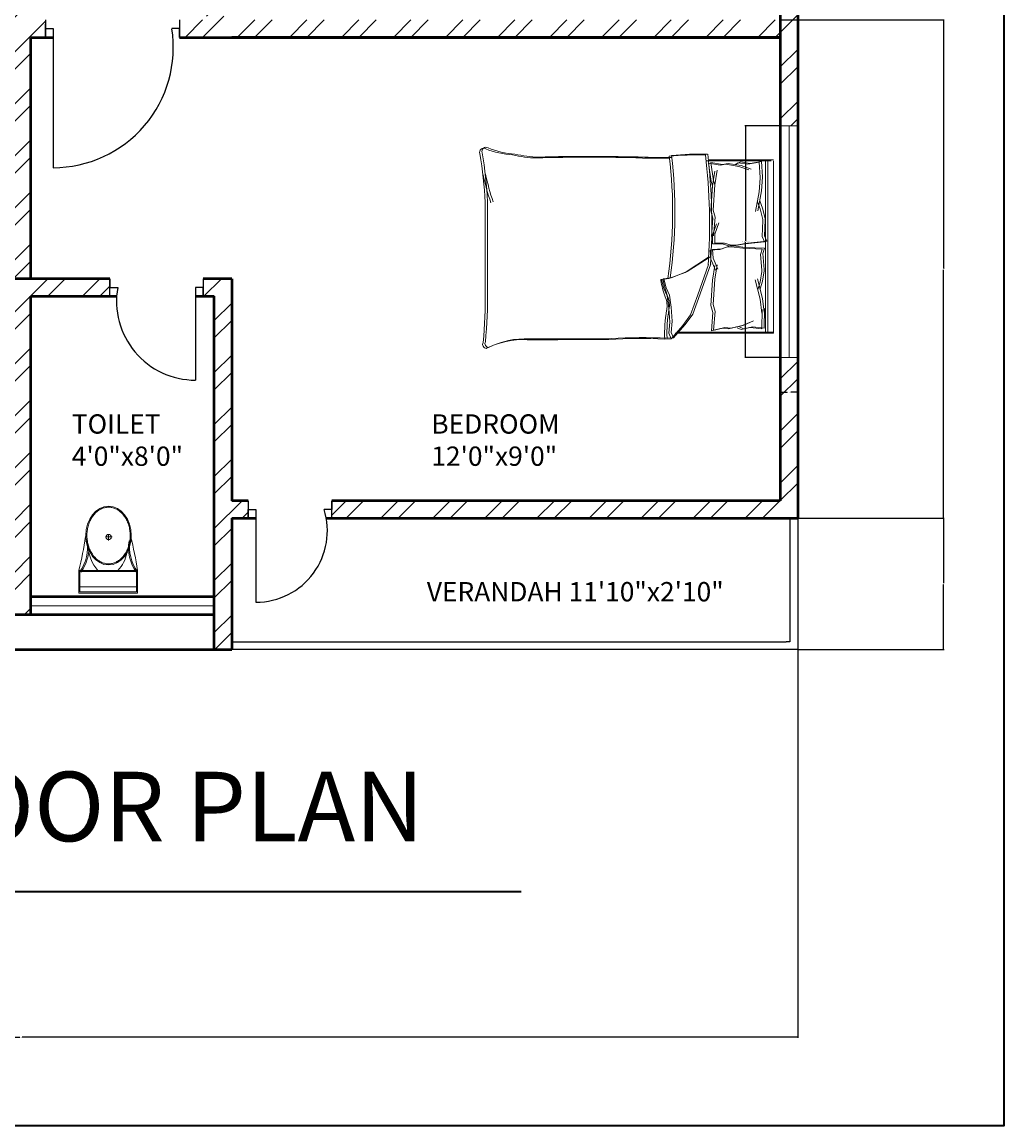
# Model space of a CAD drawing. Units: inches. Extents: x 2129 to 2642, y 1542 to 2414.
# Tile 3 of 9: x 2388 to 2642, y 1542 to 1828. Entities that reach past the tile are written whole.
import ezdxf

# ---------------------------------------------------------------- set-up
doc = ezdxf.new("R2010")
doc.units = ezdxf.units.IN
for name, color, linetype, lineweight in [('A-ANNO-DIMS', 2, 'Continuous', 18), ('A-ANNO-TITL', 7, 'Continuous', 35), ('A-ANNO-TTLB', 7, 'Continuous', 35), ('A-AREA-IDEN', 7, 'Continuous', 18), ('A-DOOR', 3, 'Continuous', 25), ('A-FLOR-FIXT', 9, 'Continuous', 18), ('A-FLOR-RAIL', 80, 'Continuous', 25), ('A-FURN', 8, 'Continuous', 18), ('A-GLAZ', 4, 'Continuous', 18), ('A-WALL', 7, 'Continuous', 50), ('A-WALL-PATT', 252, 'Continuous', 13)]:
    doc.layers.add(name, color=color, linetype=linetype, lineweight=lineweight)
doc.styles.get("Standard").update_dxf_attribs({"font": 'arial.ttf'})
doc.dimstyles.get("Standard").update_dxf_attribs({"dimtxt": 0.18, "dimasz": 0.18, "dimexe": 0.18, "dimexo": 0.0625, "dimgap": 0.09, "dimtad": 0, "dimtih": 1, "dimtoh": 1, "dimdec": 4, "dimzin": 0, "dimdsep": 46, "dimtxsty": 'Standard', "dimcen": 0.09, "dimadec": 0, "dimazin": 0, "dimtfac": 1, "dimtdec": 4, "dimtofl": 0, "dimtmove": 0, "dimatfit": 3, "dimfxl": 1, "dimtolj": 1, "dimtzin": 0, "dimarcsym": 0})

# ---------------------------------------------------------------- blocks, each defined once
blk = doc.blocks.new('A$C31115884')
for p, q in [((283.1, 497.7), (223.4, 497.7)), ((257.5, 466.4), (257.5, 523.2)), ((0, 200), (0, 0)), ((520, 200), (0, 200)), ((520, 0), (520, 200)), ((10, 190), (10, 10)), ((510, 190), (10, 190)), ((510, 10), (510, 190)), ((510, 54.5), (0, 54.5)), ((10, 10), (510, 10)), ((0, 0), (520, 0))]:
    blk.add_line(p, q)
blk.add_circle((255.6, 496.4), 23.6)
for centre, radius, start, end in [((2777.7, -204.6), 2807, 165.4549, 171.71327), ((3237, 905), 2807, 188.28673, 194.5451), ((-294.5, 403.3), 364.7, 324.20913, 9.34987), ((-294.5, 403.3), 374.7, 324.20913, 9.34987), ((139.5, 406.2), 293.5, 315.84364, 2.65635), ((805.8, 403.3), 374.7, 179.20365, 215.79087), ((805.8, 403.3), 364.7, 170.65013, 215.79087), ((383.6, 406.2), 293.5, 190.27735, 224.15636)]:
    blk.add_arc(centre, radius, start, end)
blk.add_ellipse((256.2, 509.9), major_axis=(0, -260.7), ratio=0.772727)
blk.add_open_spline([(256.2, 259.2), (263.1, 259.2), (270, 259.7), (287.8, 262.3), (298.7, 265.1), (319.9, 273.1), (330.2, 278.4), (350.1, 291.1), (359.7, 298.7), (377.7, 315.9), (386.2, 325.5), (401.7, 346.6), (408.8, 358.1), (421.3, 382.5), (426.8, 395.5), (435.9, 422.4), (439.5, 436.4), (444.8, 465.1), (446.5, 479.7), (447.9, 509.2), (447.6, 524), (445, 553.3), (442.7, 567.8), (436.3, 596), (432.1, 609.7), (421.9, 636), (416, 648.6), (402.5, 672.1), (395, 683), (378.6, 703), (369.8, 712.1), (351.1, 728), (341.3, 734.8), (320.9, 746.2), (310.4, 750.7), (288.9, 757.3), (278, 759.4), (256, 761), (245, 760.6), (223.1, 757.2), (212.3, 754.3), (191.1, 746.1), (180.8, 740.7), (160.9, 727.8), (151.4, 720.1), (133.5, 702.7), (125.1, 693), (109.6, 671.7), (102.6, 660.2), (90.2, 635.7), (84.9, 622.7), (76, 595.6), (72.4, 581.6), (67.2, 552.9), (65.6, 538.2), (64.4, 508.8), (64.8, 494), (67.5, 464.7), (69.9, 450.2), (76.6, 422), (80.8, 408.3), (91.1, 382.2), (97.2, 369.7), (110.8, 346.3), (118.4, 335.4), (134.8, 315.6), (143.7, 306.7), (162.4, 290.9), (172.3, 284.2), (192.8, 273), (203.3, 268.6), (224.8, 262.2), (235.8, 260.2), (249.9, 259.3), (253, 259.2), (256.2, 259.2)], degree=3, knots=[0, 0, 0, 0, 0.110105, 0.110105, 0.285049, 0.285049, 0.459994, 0.459994, 0.634938, 0.634938, 0.809882, 0.809882, 0.984827, 0.984827, 1.159771, 1.159771, 1.334715, 1.334715, 1.50966, 1.50966, 1.684604, 1.684604, 1.859549, 1.859549, 2.034493, 2.034493, 2.209437, 2.209437, 2.384382, 2.384382, 2.559326, 2.559326, 2.73427, 2.73427, 2.909215, 2.909215, 3.084159, 3.084159, 3.259103, 3.259103, 3.434048, 3.434048, 3.608992, 3.608992, 3.783936, 3.783936, 3.958881, 3.958881, 4.133825, 4.133825, 4.30877, 4.30877, 4.483714, 4.483714, 4.658658, 4.658658, 4.833603, 4.833603, 5.008547, 5.008547, 5.183491, 5.183491, 5.358436, 5.358436, 5.53338, 5.53338, 5.708324, 5.708324, 5.883269, 5.883269, 6.058213, 6.058213, 6.233158, 6.233158, 6.283185, 6.283185, 6.283185, 6.283185])
blk = doc.blocks.new('BED-DOUBLE')
for p, q in [((3.24, 59.14), (3.24, 76.05)), ((3.24, 74.61), (47.87, 74.61)), ((3.25, 59.14), (3.25, 76.05)), ((3.25, 74.61), (47.87, 74.61)), ((48.08, 76.05), (3.46, 76.05)), ((3.46, 58.54), (3.46, 75.45)), ((3.46, 58.54), (3.46, 75.45)), ((47.87, 76.05), (47.87, 51.2)), ((47.87, 76.05), (47.87, 51.2)), ((48.08, 76.05), (48.08, 75.45)), ((48.08, 75.45), (48.08, 50.6)), ((48.08, 75.45), (48.08, 50.6)), ((3.46, 74.02), (48.08, 74.02)), ((3.46, 74.02), (48.08, 74.02)), ((3.64, 72.93), (7.64, 73.24)), ((3.64, 72.93), (7.64, 73.24)), ((3.64, 72.95), (4.18, 69.98)), ((3.64, 72.95), (4.18, 69.98)), ((3.85, 72.33), (7.85, 72.64)), ((3.85, 72.33), (7.85, 72.64)), ((3.85, 72.35), (4.39, 69.38)), ((3.85, 72.35), (4.39, 69.38)), ((7.64, 73.24), (7.74, 73.22)), ((7.64, 73.24), (7.74, 73.22)), ((7.74, 73.22), (11.31, 72.95)), ((7.74, 73.22), (11.31, 72.95)), ((7.85, 72.64), (7.95, 72.62)), ((7.85, 72.64), (7.95, 72.62)), ((7.95, 72.62), (11.52, 72.35)), ((7.95, 72.62), (11.52, 72.35)), ((11.31, 72.95), (16.44, 72.01)), ((11.31, 72.95), (16.44, 72.01)), ((11.52, 72.35), (16.65, 71.41)), ((11.52, 72.35), (16.65, 71.41)), ((13.87, 72.55), (15.76, 73.22)), ((13.87, 72.55), (15.76, 73.22)), ((14.08, 71.95), (15.97, 72.62)), ((14.08, 71.95), (15.97, 72.62)), ((15.76, 73.22), (18.46, 73.9)), ((15.76, 73.22), (18.46, 73.9)), ((15.97, 72.62), (18.67, 73.3)), ((15.97, 72.62), (18.67, 73.3)), ((18.46, 73.9), (18.76, 73.9)), ((18.46, 73.9), (18.76, 73.9)), ((18.67, 73.3), (18.97, 73.3)), ((18.67, 73.3), (18.97, 73.3)), ((18.76, 73.9), (22.91, 73.76)), ((18.76, 73.9), (22.91, 73.76)), ((18.97, 73.3), (23.12, 73.16)), ((18.97, 73.3), (23.12, 73.16)), ((22.91, 73.76), (24.26, 74.3)), ((22.91, 73.76), (24.26, 74.3)), ((23.12, 73.16), (24.47, 73.7)), ((23.12, 73.16), (24.47, 73.7)), ((24.26, 74.3), (24.8, 69.31)), ((24.26, 74.3), (24.8, 69.31)), ((24.47, 73.7), (25.01, 68.71)), ((24.47, 73.7), (25.01, 68.71)), ((26.12, 73.72), (25.9, 68.7)), ((26.12, 73.72), (25.9, 68.7)), ((26.34, 73.12), (26.11, 68.1)), ((26.34, 73.12), (26.11, 68.1)), ((27.5, 73.27), (26.12, 73.72)), ((27.5, 73.27), (26.12, 73.72)), ((27.72, 72.67), (26.34, 73.12)), ((27.72, 72.67), (26.34, 73.12)), ((31.64, 73.66), (27.5, 73.27)), ((31.64, 73.66), (27.5, 73.27)), ((31.85, 73.06), (27.72, 72.67)), ((31.85, 73.06), (27.72, 72.67)), ((31.94, 73.68), (31.64, 73.66)), ((31.94, 73.68), (31.64, 73.66)), ((32.15, 73.08), (31.85, 73.06)), ((32.15, 73.08), (31.85, 73.06)), ((34.68, 73.17), (31.94, 73.68)), ((34.67, 73.17), (31.94, 73.68)), ((34.89, 72.58), (32.15, 73.08)), ((34.89, 72.58), (32.15, 73.08)), ((39.14, 73.18), (34.08, 71.92)), ((39.14, 73.18), (34.08, 71.92)), ((39.35, 72.58), (34.29, 71.32)), ((39.35, 72.58), (34.29, 71.32)), ((36.6, 72.62), (34.67, 73.17)), ((36.6, 72.62), (34.68, 73.17)), ((36.82, 72.02), (34.89, 72.58)), ((36.82, 72.02), (34.89, 72.58)), ((42.68, 73.67), (39.14, 73.18)), ((42.68, 73.67), (39.14, 73.18)), ((42.9, 73.08), (39.35, 72.58)), ((42.9, 73.08), (39.35, 72.58)), ((46.79, 73.66), (41.75, 73.75)), ((41.75, 73.75), (42.68, 73.67)), ((46.79, 73.66), (41.75, 73.75)), ((41.75, 73.75), (42.68, 73.67)), ((47.01, 73.06), (41.96, 73.15)), ((41.96, 73.15), (42.9, 73.08)), ((47.01, 73.06), (41.96, 73.15)), ((41.96, 73.15), (42.9, 73.08)), ((46.79, 73.66), (46.44, 70.66)), ((46.79, 73.66), (46.44, 70.66)), ((47.01, 73.06), (46.65, 70.06)), ((47.01, 73.06), (46.65, 70.06)), ((4.18, 69.98), (3.77, 67.55)), ((4.18, 69.98), (3.77, 67.55)), ((4.39, 69.38), (3.98, 66.95)), ((4.39, 69.38), (3.99, 66.95)), ((4.72, 67.69), (5.66, 70.25)), ((4.72, 67.69), (5.66, 70.25)), ((4.93, 67.09), (5.87, 69.65)), ((4.93, 67.09), (5.87, 69.65)), ((24.8, 69.31), (25.34, 66.34)), ((24.8, 69.31), (25.34, 66.34)), ((25.01, 68.71), (25.55, 65.74)), ((25.01, 68.71), (25.55, 65.74)), ((25.9, 68.7), (25.54, 65.7)), ((25.9, 68.7), (25.54, 65.7)), ((46.04, 68.34), (44.94, 70.84)), ((46.04, 68.34), (44.94, 70.84)), ((46.26, 67.74), (45.15, 70.24)), ((46.26, 67.74), (45.15, 70.24)), ((46.44, 70.66), (46.99, 68.26)), ((46.44, 70.66), (46.99, 68.26)), ((46.65, 70.06), (47.21, 67.66)), ((46.65, 70.06), (47.21, 67.66)), ((3.77, 67.55), (4.31, 66.61)), ((3.77, 67.55), (4.31, 66.61)), ((3.98, 66.95), (4.52, 66.01)), ((3.99, 66.95), (4.53, 66.01)), ((4.18, 64.31), (4.72, 67.69)), ((4.18, 64.31), (4.72, 67.69)), ((4.39, 63.71), (4.93, 67.09)), ((4.39, 63.71), (4.93, 67.09)), ((25.34, 66.34), (25.34, 65.12)), ((25.34, 66.34), (25.34, 65.12)), ((25.55, 65.74), (25.55, 64.52)), ((25.55, 65.74), (25.55, 64.52)), ((26.11, 68.1), (25.76, 65.11)), ((26.11, 68.1), (25.76, 65.11)), ((46.79, 65), (46.04, 68.34)), ((46.79, 65), (46.04, 68.34)), ((47.01, 64.41), (46.26, 67.74)), ((47.01, 64.41), (46.26, 67.74)), ((46.99, 68.26), (46.51, 67.28)), ((46.99, 68.26), (46.51, 67.28)), ((47.21, 67.66), (46.73, 66.69)), ((47.21, 67.66), (46.73, 66.69)), ((4.45, 62.82), (4.18, 64.31)), ((4.45, 62.82), (4.18, 64.31)), ((4.66, 62.23), (4.39, 63.71)), ((4.66, 62.23), (4.39, 63.71)), ((25.34, 65.12), (24.8, 63.36)), ((25.34, 65.12), (24.8, 63.36)), ((24.8, 63.36), (24.8, 60.86)), ((24.8, 63.36), (24.8, 60.86)), ((25.55, 64.52), (25.01, 62.77)), ((25.55, 64.52), (25.01, 62.77)), ((25.54, 65.7), (25.62, 64.49)), ((25.54, 65.7), (25.62, 64.49)), ((25.62, 64.49), (26.27, 62.77)), ((25.62, 64.49), (26.27, 62.77)), ((25.76, 65.11), (25.83, 63.89)), ((25.76, 65.11), (25.83, 63.89)), ((25.83, 63.89), (26.48, 62.18)), ((25.83, 63.89), (26.48, 62.18)), ((46.62, 63.5), (46.79, 65)), ((46.62, 63.5), (46.79, 65)), ((47.34, 60.57), (46.62, 63.5)), ((47.34, 60.57), (46.62, 63.5)), ((46.83, 62.91), (47.01, 64.41)), ((46.83, 62.91), (47.01, 64.41)), ((47.55, 59.98), (46.83, 62.91)), ((47.55, 59.98), (46.83, 62.91)), ((3.91, 59.85), (4.45, 62.82)), ((3.91, 59.85), (4.45, 62.82)), ((8.67, 60.53), (3.91, 59.85)), ((8.67, 60.53), (3.91, 59.85)), ((4.12, 59.26), (4.66, 62.23)), ((4.12, 59.26), (4.66, 62.23)), ((5.96, 61.45), (9.72, 60.83)), ((5.96, 61.45), (9.72, 60.83)), ((6.17, 60.86), (9.94, 60.23)), ((6.17, 60.86), (9.94, 60.23)), ((9.72, 60.83), (8.67, 60.53)), ((9.72, 60.83), (8.67, 60.53)), ((9.94, 60.23), (8.88, 59.93)), ((9.94, 60.23), (8.88, 59.93)), ((9.72, 60.83), (16.27, 60.43)), ((9.72, 60.83), (16.27, 60.43)), ((9.94, 60.23), (16.48, 59.83)), ((9.94, 60.23), (16.48, 59.83)), ((16.27, 60.43), (18.1, 60.95)), ((16.27, 60.43), (18.1, 60.95)), ((16.48, 59.83), (18.31, 60.35)), ((16.48, 59.83), (18.31, 60.35)), ((18.1, 60.95), (22.89, 60.57)), ((18.1, 60.95), (22.89, 60.57)), ((18.31, 60.35), (23.11, 59.98)), ((18.31, 60.35), (23.1, 59.98)), ((22.51, 60.86), (19.57, 61.88)), ((22.51, 60.86), (19.57, 61.88)), ((22.72, 60.26), (19.78, 61.28)), ((22.72, 60.26), (19.78, 61.28)), ((24.8, 60.86), (22.51, 60.86)), ((24.8, 60.86), (22.51, 60.86)), ((25.01, 60.26), (22.72, 60.26)), ((25.01, 60.26), (22.72, 60.26)), ((25.01, 62.77), (25.01, 60.26)), ((25.01, 62.77), (25.01, 60.26)), ((26.27, 62.77), (26.42, 60.27)), ((26.27, 62.77), (26.42, 60.27)), ((26.42, 60.27), (28.71, 60.42)), ((26.42, 60.27), (28.71, 60.42)), ((26.48, 62.18), (26.64, 59.68)), ((26.48, 62.18), (26.64, 59.68)), ((28.71, 60.42), (31.58, 61.62)), ((28.71, 60.42), (31.58, 61.62)), ((28.93, 59.82), (31.79, 61.02)), ((28.93, 59.82), (31.79, 61.02)), ((30.41, 61.45), (34.17, 60.83)), ((30.41, 61.45), (34.17, 60.83)), ((30.62, 60.86), (34.39, 60.23)), ((30.62, 60.86), (34.38, 60.23)), ((34.17, 60.83), (40.72, 60.43)), ((34.17, 60.83), (40.72, 60.43)), ((34.38, 60.23), (40.93, 59.83)), ((34.39, 60.23), (40.93, 59.83)), ((40.72, 60.43), (42.55, 60.95)), ((40.72, 60.43), (42.55, 60.95)), ((40.93, 59.83), (42.76, 60.35)), ((40.93, 59.83), (42.76, 60.35)), ((42.55, 60.95), (47.34, 60.57)), ((42.55, 60.95), (47.34, 60.57)), ((42.76, 60.35), (47.55, 59.98)), ((42.76, 60.35), (47.55, 59.98)), ((8.88, 59.93), (4.12, 59.26)), ((8.88, 59.93), (4.12, 59.26)), ((26.64, 59.68), (28.93, 59.82)), ((26.64, 59.68), (28.93, 59.82)), ((28.25, 59.82), (32.17, 53.75)), ((28.25, 59.82), (32.17, 53.75)), ((28.47, 59.22), (32.38, 53.16)), ((28.47, 59.22), (32.38, 53.16)), ((37.95, 57.08), (30.17, 59.82)), ((37.95, 57.08), (30.17, 59.82)), ((38.16, 56.48), (30.38, 59.22)), ((38.16, 56.48), (30.38, 59.22)), ((43.16, 55.2), (37.95, 57.08)), ((43.16, 55.2), (37.95, 57.08)), ((43.37, 54.6), (38.16, 56.48)), ((43.37, 54.6), (38.16, 56.48)), ((45.91, 53.17), (43.16, 55.2)), ((45.91, 53.17), (43.16, 55.2)), ((46.12, 52.58), (43.37, 54.6)), ((46.12, 52.58), (43.37, 54.6)), ((32.17, 53.75), (33.76, 49.56)), ((32.17, 53.75), (33.76, 49.56)), ((32.38, 53.16), (33.97, 48.96)), ((32.38, 53.16), (33.97, 48.96)), ((49.37, 50.14), (45.91, 53.17)), ((49.36, 50.14), (45.91, 53.17)), ((49.58, 49.54), (46.12, 52.58)), ((49.58, 49.54), (46.12, 52.58)), ((33.76, 49.56), (34.05, 47.68)), ((33.76, 49.56), (34.05, 47.68)), ((33.97, 48.96), (34.26, 47.09)), ((33.97, 48.96), (34.26, 47.09)), ((36.36, 48.26), (38.24, 49.13)), ((36.36, 48.26), (38.24, 49.13)), ((38.24, 49.13), (41.42, 49.56)), ((38.24, 49.13), (41.42, 49.56)), ((38.45, 48.53), (41.64, 48.96)), ((38.45, 48.53), (41.64, 48.96)), ((41.42, 49.56), (45.04, 49.85)), ((41.42, 49.56), (45.04, 49.85)), ((41.64, 48.96), (45.25, 49.25)), ((41.64, 48.96), (45.25, 49.25)), ((45.04, 49.85), (47.93, 49.56)), ((45.04, 49.85), (47.93, 49.56)), ((45.25, 49.25), (48.14, 48.96)), ((45.25, 49.25), (48.14, 48.96)), ((47.93, 49.56), (49.37, 50.14)), ((47.93, 49.56), (49.36, 50.14)), ((48.14, 48.96), (49.58, 49.54)), ((48.14, 48.96), (49.58, 49.54)), ((49.44, 48.51), (49.36, 50.14, 3.61)), ((49.44, 48.51), (49.37, 50.14, 3.61)), ((49.65, 47.91), (49.58, 49.54, 3.61)), ((49.65, 47.91), (49.58, 49.54, 3.61)), ((34.05, 47.68), (36.36, 48.26)), ((34.05, 47.68), (36.36, 48.26)), ((34.26, 47.09), (36.57, 47.66)), ((34.26, 47.09), (36.57, 47.66)), ((36.57, 47.66), (38.45, 48.53)), ((36.57, 47.66), (38.45, 48.53)), ((14.07, 2.05), (37.05, 2.05)), ((14.07, 2.05), (37.05, 2.05)), ((14.28, 1.46), (37.26, 1.46)), ((14.28, 1.46), (37.26, 1.46))]:
    blk.add_line(p, q)
for centre, radius, start, end in [((19.94, -93.94), 154.04, 86.0865, 96.7821), ((19.94, -93.94), 154.04, 86.0865, 96.7821), ((79.52, 57.28), 77.79, 178.7218, 185.604), ((79.52, 57.28), 77.79, 178.7218, 185.604), ((79.73, 56.69), 77.79, 178.7218, 185.604), ((79.73, 56.69), 77.79, 178.7218, 185.604), ((20.16, -94.54), 154.04, 86.0865, 96.7821), ((20.16, -94.54), 154.04, 86.0865, 96.7821), ((16.58, -69.91), 120.47, 81.7845, 96.9006), ((16.58, -69.91), 120.47, 81.7845, 96.9006), ((16.79, -70.51), 120.47, 81.7845, 96.9006), ((16.79, -70.51), 120.47, 81.7845, 96.9006), ((-156.22, 46.94), 158.84, 358.4762, 1.0082), ((-156.22, 46.94), 158.84, 358.4762, 1.0082), ((-156.01, 46.34), 158.84, 358.4762, 1.0082), ((-156.01, 46.34), 158.84, 358.4762, 1.0082), ((29.09, 74.66), 27.69, 280.6617, 289.8806), ((29.09, 74.66), 27.69, 280.6617, 289.8806), ((40.85, 43.3), 5.81, 78.6608, 113.7384), ((40.85, 43.3), 5.81, 78.6608, 113.7384), ((47.93, 82.26), 33.79, 259.8763, 272.5657), ((47.93, 82.26), 33.79, 259.8763, 272.5657), ((34.21, 47.62), 0.172, 160.2464, 271.1377), ((34.21, 47.62), 0.172, 160.2464, 271.1377), ((34.42, 47.03), 0.172, 160.2464, 271.1377), ((34.42, 47.03), 0.172, 160.2464, 271.1377), ((29.3, 74.07), 27.69, 280.6617, 289.8806), ((29.3, 74.07), 27.69, 280.6617, 289.8806), ((41.06, 42.71), 5.81, 78.6608, 113.7384), ((41.06, 42.71), 5.81, 78.6608, 113.7384), ((48.14, 81.67), 33.79, 259.8763, 272.5657), ((48.14, 81.67), 33.79, 259.8763, 272.5657), ((170.19, 42.14), 120.92, 176.9791, 183.8365), ((170.19, 42.14), 120.92, 176.9791, 183.8365), ((170.4, 41.54), 120.92, 176.9791, 183.8365), ((170.4, 41.54), 120.92, 176.9791, 183.8365), ((452.7, 28.79), 450.36, 178.2277, 181.7185), ((452.7, 28.79), 450.36, 178.2277, 181.7185), ((452.91, 28.19), 450.36, 178.2277, 181.7185), ((452.91, 28.19), 450.36, 178.2277, 181.7185), ((-4210.02, 12.72), 4259.62, 0.00217, 0.28689), ((-4210.02, 12.72), 4259.62, 0.00217, 0.28689), ((-4209.81, 12.12), 4259.62, 0.00217, 0.28689), ((-4209.81, 12.12), 4259.62, 0.00217, 0.28689), ((-25.12, 15.81), 27.67, 346.0648, 358.9113), ((-25.12, 15.81), 27.67, 346.0648, 358.9113), ((-24.9, 15.21), 27.67, 346.0648, 358.9113), ((-24.9, 15.21), 27.67, 346.0648, 358.9113), ((71.11, 11.93), 21.54, 177.4714, 206.4681), ((71.11, 11.93), 21.54, 177.4714, 206.4681), ((71.33, 11.33), 21.54, 177.4714, 206.4681), ((71.32, 11.33), 21.54, 177.4714, 206.4681), ((-20.22, 10.43), 22, 337.9751, 356.652), ((-20.22, 10.43), 22, 337.9751, 356.652), ((-20.01, 9.83), 22, 337.9751, 356.652), ((-20.01, 9.83), 22, 337.9751, 356.652), ((-16.08, 98.19), 99.41, 283.3832, 287.7053), ((-16.08, 98.19), 99.41, 283.3832, 287.7053), ((-15.87, 97.59), 99.41, 283.3832, 287.7053), ((-15.87, 97.59), 99.41, 283.3832, 287.7053), ((1.02, 1.61), 1.02, 146.1736, 293.4781), ((1.02, 1.61), 1.02, 146.1736, 293.4781), ((1.23, 1.01), 1.02, 146.1736, 293.4781), ((1.23, 1.01), 1.02, 146.1736, 293.4781), ((20.01, -111.48), 113.69, 92.9958, 99.4091), ((20.01, -111.48), 113.69, 92.9958, 99.4091), ((20.22, -112.08), 113.69, 92.9958, 99.4091), ((20.22, -112.08), 113.69, 92.9958, 99.4091), ((38.43, -122.17), 124.23, 84.4998, 90.6351), ((38.43, -122.17), 124.23, 84.4998, 90.6351), ((38.64, -122.76), 124.23, 84.4998, 90.6351), ((38.64, -122.76), 124.23, 84.4998, 90.6351), ((50.81, 2.4), 1.03, 242.6588, 356.02), ((50.81, 2.4), 1.03, 242.6588, 356.02), ((51.02, 1.81), 1.03, 242.6588, 356.02), ((51.02, 1.81), 1.03, 242.6588, 356.02)]:
    blk.add_arc(centre, radius, start, end)
blk = doc.blocks.new('WIN-60-A')
for p, q in [((0, 4.5), (0, 0)), ((60, 2.25), (60, 4.5)), ((60, 4.5), (60, 0)), ((0, 0), (0, 2.25)), ((0, 2.25), (60, 2.25))]:
    blk.add_line(p, q)
blk = doc.blocks.new('*D14')
at = {"layer": 'A-ANNO-DIMS', "color": 0, "lineweight": -2, "transparency": 16777216}
for p, q in [((2584.34, 1801.35), (2575.22, 1801.35)), ((2575.4, 1801.17), (2575.4, 1771.54)), ((2575.4, 1741.53), (2575.4, 1771.17)), ((2584.34, 1741.35), (2575.22, 1741.35))]:
    blk.add_line(p, q, dxfattribs=at)
at = {"layer": 'A-ANNO-DIMS', "color": 0, "transparency": 16777216}
for points in [[(2575.37, 1801.17), (2575.43, 1801.17), (2575.4, 1801.35)], [(2575.37, 1741.53), (2575.43, 1741.53), (2575.4, 1741.35)]]:
    blk.add_solid(points, dxfattribs=at)
at = {"layer": 'Defpoints', "color": 0, "transparency": 16777216}
for p in [(2584.4, 1801.35), (2575.4, 1741.35), (2584.4, 1741.35)]:
    blk.add_point(p, dxfattribs=at)
at = {"layer": 'A-ANNO-DIMS', "color": 0, "transparency": 16777216, "insert": (2575.4, 1771.35), "char_height": 0.18, "attachment_point": 5}
blk.add_mtext('\\A1;WINDOW A 60 TYP.', dxfattribs=at)
blk = doc.blocks.new('*D15')
at = {"layer": 'A-ANNO-DIMS', "color": 0, "lineweight": -2, "transparency": 16777216}
for p, q in [((2584.4, 1741.29), (2584.4, 1732.17)), ((2588.9, 1741.29), (2588.9, 1732.17)), ((2584.58, 1732.35), (2586.2, 1732.35)), ((2588.72, 1732.35), (2587.11, 1732.35))]:
    blk.add_line(p, q, dxfattribs=at)
at = {"layer": 'A-ANNO-DIMS', "color": 0, "transparency": 16777216}
for points in [[(2584.58, 1732.38), (2584.58, 1732.32), (2584.4, 1732.35)], [(2588.72, 1732.38), (2588.72, 1732.32), (2588.9, 1732.35)]]:
    blk.add_solid(points, dxfattribs=at)
at = {"layer": 'Defpoints', "color": 0, "transparency": 16777216}
for p in [(2584.4, 1741.35), (2588.9, 1741.35), (2588.9, 1732.35)]:
    blk.add_point(p, dxfattribs=at)
at = {"layer": 'A-ANNO-DIMS', "color": 0, "transparency": 16777216, "insert": (2586.65, 1732.35), "char_height": 0.18, "attachment_point": 5}
blk.add_mtext('\\A1;5 TYP.', dxfattribs=at)
blk = doc.blocks.new('*D34')
at = {"layer": 'A-ANNO-DIMS', "color": 0, "lineweight": -2, "transparency": 16777216}
for p, q in [((2186.9, 1665.66), (2186.9, 1565.16)), ((2588.9, 1665.66), (2588.9, 1565.16)), ((2187.08, 1565.34), (2387.61, 1565.34)), ((2588.72, 1565.34), (2388.2, 1565.34))]:
    blk.add_line(p, q, dxfattribs=at)
at = {"layer": 'A-ANNO-DIMS', "color": 0, "transparency": 16777216}
for points in [[(2187.08, 1565.37), (2187.08, 1565.31), (2186.9, 1565.34)], [(2588.72, 1565.37), (2588.72, 1565.31), (2588.9, 1565.34)]]:
    blk.add_solid(points, dxfattribs=at)
at = {"layer": 'Defpoints', "color": 0, "transparency": 16777216}
for p in [(2186.9, 1665.72), (2588.9, 1665.72), (2588.9, 1565.34)]:
    blk.add_point(p, dxfattribs=at)
at = {"layer": 'A-ANNO-DIMS', "color": 0, "transparency": 16777216, "insert": (2387.9, 1565.34), "char_height": 0.18, "attachment_point": 5}
blk.add_mtext('\\A1;402', dxfattribs=at)
blk = doc.blocks.new('*D39')
at = {"layer": 'A-ANNO-DIMS', "color": 0, "lineweight": -2, "transparency": 16777216}
for p, q in [((2588.97, 1699.72), (2626.83, 1699.72)), ((2626.65, 1699.54), (2626.65, 1682.9)), ((2626.65, 1665.9), (2626.65, 1682.54)), ((2588.97, 1665.72), (2626.83, 1665.72))]:
    blk.add_line(p, q, dxfattribs=at)
at = {"layer": 'A-ANNO-DIMS', "color": 0, "transparency": 16777216}
for points in [[(2626.62, 1699.54), (2626.68, 1699.54), (2626.65, 1699.72)], [(2626.62, 1665.9), (2626.68, 1665.9), (2626.65, 1665.72)]]:
    blk.add_solid(points, dxfattribs=at)
at = {"layer": 'Defpoints', "color": 0, "transparency": 16777216}
for p in [(2588.9, 1699.72), (2626.65, 1699.72), (2588.9, 1665.72)]:
    blk.add_point(p, dxfattribs=at)
at = {"layer": 'A-ANNO-DIMS', "color": 0, "transparency": 16777216, "insert": (2626.65, 1682.72), "char_height": 0.18, "attachment_point": 5}
blk.add_mtext('\\A1;34', dxfattribs=at)
blk = doc.blocks.new('*D40')
at = {"layer": 'A-ANNO-DIMS', "color": 0, "lineweight": -2, "transparency": 16777216}
for p, q in [((2584.47, 1828.72), (2626.83, 1828.72)), ((2626.65, 1828.54), (2626.65, 1764.4)), ((2626.65, 1699.9), (2626.65, 1764.04)), ((2588.97, 1699.72), (2626.83, 1699.72))]:
    blk.add_line(p, q, dxfattribs=at)
at = {"layer": 'A-ANNO-DIMS', "color": 0, "transparency": 16777216}
for points in [[(2626.62, 1828.54), (2626.68, 1828.54), (2626.65, 1828.72)], [(2626.62, 1699.9), (2626.68, 1699.9), (2626.65, 1699.72)]]:
    blk.add_solid(points, dxfattribs=at)
at = {"layer": 'Defpoints', "color": 0, "transparency": 16777216}
for p in [(2584.4, 1828.72), (2626.65, 1828.72), (2588.9, 1699.72)]:
    blk.add_point(p, dxfattribs=at)
at = {"layer": 'A-ANNO-DIMS', "color": 0, "transparency": 16777216, "insert": (2626.65, 1764.22), "char_height": 0.18, "attachment_point": 5}
blk.add_mtext('\\A1;129', dxfattribs=at)

msp = doc.modelspace()

# ---------------------------------------------------------------- hatches: boundary and pattern name
at = {"layer": 'A-WALL-PATT'}
h = msp.add_hatch(dxfattribs=at)
h.set_pattern_fill('ANSI32', color=256)
h.paths.add_polyline_path([(2306.2606, 2305.9717), (2306.2606, 2308.2217), (2276.3515, 2308.2217), (2276.3515, 2303.7217), (2306.2606, 2303.7217)])
h.paths.add_polyline_path([(2216.3515, 2305.9717), (2216.3515, 2308.2217), (2186.9043, 2308.2217), (2186.9043, 2278.1696), (2191.4043, 2278.1696), (2191.4043, 2303.7217), (2216.3515, 2303.7217)])
h.paths.add_polyline_path([(2339.9043, 2335.7217), (2362.1938, 2335.7217), (2362.1938, 2340.2217), (2335.4043, 2340.2217), (2335.4043, 2308.2217), (2329.3487, 2308.2217), (2329.3487, 2305.9717), (2329.3487, 2303.7217), (2335.4043, 2303.7217), (2335.4043, 2186.7217), (2329.4345, 2186.7217), (2329.4345, 2182.2217), (2335.4043, 2182.2217), (2335.4043, 2174.7178), (2339.9043, 2174.7178), (2339.9043, 2182.2217), (2339.9043, 2303.7217)])
h.paths.add_polyline_path([(2440.4043, 2340.2217), (2411.654, 2340.2217), (2411.654, 2335.7217), (2435.9043, 2335.7217), (2435.9043, 2303.7217), (2435.9043, 2182.2217), (2435.9043, 2174.1935), (2438.1543, 2174.1935), (2440.4043, 2174.1935), (2440.4043, 2182.2217), (2444.653, 2182.2217), (2444.653, 2184.4717), (2444.653, 2186.7217), (2440.4043, 2186.7217), (2440.4043, 2303.7217), (2445.8547, 2303.7217), (2445.8547, 2308.2217), (2440.4043, 2308.2217)])
h.paths.add_polyline_path([(2498.2381, 2308.2217), (2470.3901, 2308.2217), (2470.3901, 2303.7217), (2498.2381, 2303.7217), (2498.2381, 2305.9717)])
h.paths.add_polyline_path([(2588.9043, 2308.2217), (2586.9043, 2308.2217), (2558.2381, 2308.2217), (2558.2381, 2303.7217), (2584.4043, 2303.7217), (2584.4043, 2279.1087), (2588.9043, 2279.1087)])
h.paths.add_polyline_path([(2588.9043, 2219.1087), (2584.4043, 2219.1087), (2584.4043, 2186.7217), (2478.0667, 2186.7217), (2478.0667, 2182.2217), (2584.4043, 2182.2217), (2584.4043, 2157.7883), (2588.9043, 2157.7883)])
h.paths.add_polyline_path([(2588.9043, 2097.7883), (2584.6063, 2097.7883), (2584.6063, 2075.5462, -0.09241561), (2584.4043, 2074.4627), (2584.4043, 2064.2217), (2495.9043, 2064.2217), (2495.9043, 2040.4611), (2500.4043, 2040.4611), (2500.4043, 2059.7217), (2584.4043, 2059.7217), (2584.4043, 2052.2164), (2588.9043, 2052.2164)])
h.paths.add_polyline_path([(2588.9043, 2028.2164), (2584.4043, 2028.2164), (2584.4043, 2011.7217), (2500.4043, 2011.7217), (2500.4043, 2015.243), (2498.1543, 2015.243), (2495.9043, 2015.243), (2495.9043, 2007.2217), (2495.9043, 2003.7597), (2500.4043, 2003.7597), (2500.4043, 2007.2217), (2584.4043, 2007.2217), (2584.4043, 1992.1997), (2588.9043, 1992.1997)])
h.paths.add_polyline_path([(2588.9043, 1956.1997), (2584.4043, 1956.1997), (2584.4043, 1941.2217), (2500.4043, 1941.2217), (2500.4043, 1985.1493), (2498.1543, 1985.1493), (2495.9043, 1985.1493), (2495.9043, 1941.2217), (2435.9043, 1941.2217), (2435.9043, 1930.3963), (2440.4043, 1930.3963), (2440.4043, 1936.7217), (2584.4043, 1936.7217), (2584.4043, 1909.8406), (2588.9043, 1909.8406)])
h.paths.add_polyline_path([(2588.9043, 1849.8406), (2584.4043, 1849.8406), (2584.4043, 1801.3526), (2588.9043, 1801.3526)])
h.paths.add_polyline_path([(2584.4043, 1828.7217), (2495.9043, 1828.7217), (2440.4043, 1828.7217), (2440.4043, 1905.2159), (2438.1543, 1905.2159), (2435.9043, 1905.2159), (2435.9043, 1828.7217), (2428.9101, 1828.7217), (2428.9101, 1824.2217), (2584.4043, 1824.2217)])
h.paths.add_polyline_path([(2588.9043, 1741.3526), (2584.4043, 1741.3526), (2584.4043, 1704.2217), (2468.3173, 1704.2217), (2468.3173, 1701.9717), (2468.3173, 1699.7217), (2588.9043, 1699.7217)])
h.paths.add_polyline_path([(2442.4043, 1761.7217), (2435.0216, 1761.7217), (2435.0216, 1757.2217), (2437.9043, 1757.2217), (2437.9043, 1665.7217), (2442.4043, 1665.7217), (2442.4043, 1667.7217), (2442.4043, 1699.7217), (2446.6907, 1699.7217), (2446.6907, 1701.9717), (2446.6907, 1704.2217), (2442.4043, 1704.2217)])
h.paths.add_polyline_path([(2390.4043, 1757.2217), (2410.8996, 1757.2217), (2410.8996, 1761.7217), (2360.1741, 1761.7217), (2360.1741, 1759.4717), (2360.1741, 1757.2217), (2385.9043, 1757.2217), (2385.9043, 1674.8326), (2390.4043, 1674.8326)])
h.paths.add_polyline_path([(2337.9043, 1757.2217), (2340.3592, 1757.2217), (2340.3592, 1759.4717), (2340.3592, 1761.7217), (2333.4043, 1761.7217), (2333.4043, 1704.2217), (2327.381, 1704.2217), (2327.381, 1701.9717), (2327.381, 1699.7217), (2333.4043, 1699.7217), (2333.4043, 1665.7217), (2337.9043, 1665.7217)])
h.paths.add_polyline_path([(2191.4043, 1743.4804), (2186.9043, 1743.4804), (2186.9043, 1699.7217), (2188.9043, 1699.7217), (2191.4043, 1699.7217), (2306.5617, 1699.7217), (2306.5617, 1704.2217), (2191.4043, 1704.2217)])
h.paths.add_polyline_path([(2191.4043, 1859.8992), (2186.9043, 1859.8992), (2186.9043, 1803.4804), (2189.1543, 1803.4804), (2191.4043, 1803.4804)])
h.paths.add_polyline_path([(2352.5445, 1828.7217), (2191.4043, 1828.7217), (2191.4043, 1824.2217), (2333.4043, 1824.2217), (2352.5445, 1824.2217), (2352.5445, 1826.4717)])
h.paths.add_polyline_path([(2390.4043, 2085.328), (2385.9043, 2085.328), (2385.9043, 1828.7217), (2381.9668, 1828.7217), (2381.9668, 1826.4717), (2381.9668, 1824.2217), (2385.9043, 1824.2217), (2385.9043, 1761.7217), (2390.4043, 1761.7217), (2390.4043, 1824.2217), (2394.1868, 1824.2217), (2394.1868, 1827.6339), (2394.1868, 1828.7217), (2390.4043, 1828.7217)])
h.paths.add_polyline_path([(2339.9043, 1941.2217), (2335.4043, 1941.2217), (2279.9043, 1941.2217), (2279.9043, 1981.3432), (2277.6543, 1981.3432), (2275.4043, 1981.3432), (2275.4043, 1941.2217), (2191.4043, 1941.2217), (2191.4043, 1958.1079), (2186.9043, 1958.1079), (2186.9043, 1919.8992), (2189.1543, 1919.8992), (2191.4043, 1919.8992), (2191.4043, 1936.7217), (2279.9043, 1936.7217), (2335.4043, 1936.7217), (2335.4043, 1931.1382), (2339.9043, 1931.1382)])
h.paths.add_polyline_path([(2339.9043, 1902.7544), (2337.6543, 1902.7544), (2335.4043, 1902.7544), (2335.4043, 1828.7217), (2339.9043, 1828.7217)])
h.paths.add_polyline_path([(2279.9043, 2015.263), (2277.6543, 2015.263), (2275.4043, 2015.263), (2275.4043, 2011.7217), (2191.4043, 2011.7217), (2191.4043, 2026.6781), (2186.9043, 2026.6781), (2186.9043, 1994.1079), (2189.1543, 1994.1079), (2191.4043, 1994.1079), (2191.4043, 2007.2217), (2275.4043, 2007.2217), (2275.4043, 2003.2288), (2279.9043, 2003.2288), (2279.9043, 2007.2217)])
h.paths.add_polyline_path([(2296.0216, 2186.7217), (2191.4043, 2186.7217), (2191.4043, 2218.1696), (2186.9043, 2218.1696), (2186.9043, 2158.4509), (2191.4043, 2158.4509), (2191.4043, 2182.2217), (2296.0216, 2182.2217), (2296.0216, 2184.4717)])
h.paths.add_polyline_path([(2191.4043, 2098.4509), (2189.1543, 2098.4509), (2186.9043, 2098.4509), (2186.9043, 2050.6781), (2189.0487, 2050.6781), (2191.4043, 2050.6781), (2191.4043, 2059.7217), (2275.4043, 2059.7217), (2275.4043, 2038.4133), (2279.9043, 2038.4133), (2279.9043, 2064.2217), (2191.4043, 2064.2217)])
h.paths.add_polyline_path([(2268.3923, 1605.9386), (2516.3159, 1605.9386), (2516.3159, 1643.0314), (2268.3923, 1643.0314)], flags=9)
h.paths.add_polyline_path([(2399.6079, 1710.4489), (2428.8405, 1710.4489), (2428.8405, 1729.1062), (2399.6079, 1729.1062)], flags=9)
h.paths.add_polyline_path([(2342.1483, 1708.9956), (2371.3809, 1708.9956), (2371.3809, 1727.653), (2342.1483, 1727.653)], flags=9)
h.paths.add_polyline_path([(2200.7404, 1677.2519), (2282.3059, 1677.2519), (2282.3059, 1687.5555), (2200.7404, 1687.5555)], flags=9)
h.paths.add_polyline_path([(2209.8153, 1704.7448), (2250.627, 1704.7448), (2250.627, 1723.4021), (2209.8153, 1723.4021)], flags=25)
h.paths.add_polyline_path([(2213.9996, 1911.284), (2252.84, 1911.284), (2252.84, 1929.9413), (2213.9996, 1929.9413)], flags=9)
h.paths.add_polyline_path([(2210.8865, 1962.0987), (2244.0447, 1962.0987), (2244.0447, 1980.7561), (2210.8865, 1980.7561)], flags=25)
h.paths.add_polyline_path([(2219.0745, 2037.6131), (2248.2321, 2037.6131), (2248.2321, 2056.2705), (2219.0745, 2056.2705)], flags=9)
h.paths.add_polyline_path([(2379.9702, 2099.0686), (2409.3767, 2099.0686), (2409.3767, 2117.7259), (2379.9702, 2117.7259)], flags=9)
h.paths.add_polyline_path([(2375.9312, 2160.3752), (2405.3173, 2160.3752), (2405.3173, 2179.0325), (2375.9312, 2179.0325)], flags=9)
h.paths.add_polyline_path([(2269.5058, 2112.1824), (2310.3175, 2112.1824), (2310.3175, 2130.8397), (2269.5058, 2130.8397)], flags=9)
h.paths.add_polyline_path([(2209.6567, 2193.667), (2248.4971, 2193.667), (2248.4971, 2212.3243), (2209.6567, 2212.3243)], flags=25)
h.paths.add_polyline_path([(2491.6289, 1675.447), (2573.1944, 1675.447), (2573.1944, 1685.7506), (2491.6289, 1685.7506)], flags=9)
h.paths.add_polyline_path([(2492.0585, 1710.4489), (2530.8989, 1710.4489), (2530.8989, 1729.1062), (2492.0585, 1729.1062)], flags=25)
h.paths.add_polyline_path([(2495.6634, 1908.8646), (2534.5038, 1908.8646), (2534.5038, 1927.522), (2495.6634, 1927.522)], flags=9)
h.paths.add_polyline_path([(2516.7779, 1955.9942), (2549.9362, 1955.9942), (2549.9362, 1974.6516), (2516.7779, 1974.6516)], flags=25)
h.paths.add_polyline_path([(2509.7444, 2034.6896), (2538.902, 2034.6896), (2538.902, 2053.347), (2509.7444, 2053.347)], flags=9)
h.paths.add_polyline_path([(2467.8454, 2111.9593), (2508.6571, 2111.9593), (2508.6571, 2130.6167), (2467.8454, 2130.6167)], flags=9)
h.paths.add_polyline_path([(2528.5267, 2189.1742), (2567.3671, 2189.1742), (2567.3671, 2207.8316), (2528.5267, 2207.8316)], flags=25)
h.paths.add_polyline_path([(2483.7603, 2319.9841), (2557.5563, 2319.9841), (2557.5563, 2330.2877), (2483.7603, 2330.2877)], flags=9)
h.paths.add_polyline_path([(2204.078, 2317.0445), (2277.874, 2317.0445), (2277.874, 2327.3481), (2204.078, 2327.3481)], flags=9)

# ---------------------------------------------------------------- linework, layer by layer
at = {"layer": 'A-ANNO-TITL'}
for p in [(2268.1427, 1603.0854), (2517.3006, 1603.0854)]:
    msp.add_line(p, (2517.3006, 1603.0854), dxfattribs=at)
at = {"layer": 'A-ANNO-TTLB'}
msp.add_lwpolyline([(2129.4387, 2413.7704), (2642.2731, 2413.7704), (2642.2731, 1542.3836), (2129.4387, 1542.3836)], close=True, dxfattribs=at)
at = {"layer": 'A-DOOR'}
for p, q in [((2394.1868, 1828.7217), (2394.1868, 1824.2217)), ((2394.1868, 1824.2217), (2394.1868, 1827.6339)), ((2394.1868, 1827.6339), (2394.1868, 1826.4717)), ((2394.1868, 1826.4717), (2396.1868, 1826.4717)), ((2396.1868, 1826.4717), (2396.1868, 1790.4717)), ((2428.9101, 1826.4717), (2426.9101, 1826.4717)), ((2428.9101, 1828.7217), (2428.9101, 1824.2217)), ((2428.9101, 1824.2217), (2428.9101, 1826.4717)), ((2410.8996, 1757.2217), (2410.8996, 1761.7217)), ((2410.8996, 1761.7217), (2410.8996, 1759.4717)), ((2435.0216, 1761.7217), (2435.0216, 1757.2217)), ((2410.8996, 1759.4717), (2412.8996, 1759.4717)), ((2435.0216, 1759.4717), (2433.0216, 1759.4717)), ((2433.0216, 1759.4717), (2433.0216, 1735.4717)), ((2435.0216, 1757.2217), (2435.0216, 1759.4717)), ((2435.0216, 1759.4717), (2435.0216, 1759.4717)), ((2446.6907, 1704.2217), (2446.6907, 1699.7217)), ((2468.3173, 1699.7217), (2468.3173, 1704.2217)), ((2468.3173, 1704.2217), (2468.3173, 1701.9717)), ((2446.6907, 1699.7217), (2446.6907, 1701.9717)), ((2446.6907, 1701.9717), (2448.6907, 1701.9717)), ((2448.6907, 1701.9717), (2448.6907, 1677.9717)), ((2468.3173, 1701.9717), (2466.3173, 1701.9717))]:
    msp.add_line(p, q, dxfattribs=at)
for centre, radius, start, end in [((2396.1868, 1821.5816), 31.1099, 270, 9.043613), ((2433.0216, 1755.907), 20.4353, 169.95407, 270), ((2448.6907, 1696.4445), 18.4728, 270, 17.409965)]:
    msp.add_arc(centre, radius, start, end, dxfattribs=at)
at = {"layer": 'A-FLOR-RAIL'}
for p, q in [((2586.9043, 1699.7217), (2586.9043, 1667.7217)), ((2588.9043, 1699.7217), (2588.9043, 1665.7217)), ((2442.4043, 1665.7217), (2442.4043, 1667.7217)), ((2442.4043, 1667.7217), (2585.9043, 1667.7217)), ((2586.9043, 1667.7217), (2585.9043, 1667.7217)), ((2587.9043, 1665.7217), (2442.4043, 1665.7217)), ((2588.9043, 1665.7217), (2587.9043, 1665.7217)), ((2588.9043, 1665.7217), (2588.9043, 1665.7217))]:
    msp.add_line(p, q, dxfattribs=at)
at = {"layer": 'A-GLAZ'}
for p, q in [((2584.4043, 1801.3526), (2584.4043, 1801.3526)), ((2390.4043, 1677.0587), (2437.9043, 1677.0587))]:
    msp.add_line(p, q, dxfattribs=at)
at = {"layer": 'A-WALL'}
for p, q in [((2588.9043, 2308.2217), (2588.9043, 1699.7217)), ((2584.4043, 1936.7217), (2584.4043, 1704.2217)), ((2390.4043, 1761.7217), (2390.4043, 1824.2217)), ((2390.4043, 1824.2217), (2396.1868, 1824.2217)), ((2428.9101, 1824.2217), (2584.4043, 1824.2217)), ((2584.4043, 1824.2217), (2442.4043, 1824.2217)), ((2584.4043, 1824.2217), (2584.4043, 1704.2217)), ((2410.8996, 1761.7217), (2360.1741, 1761.7217)), ((2442.4043, 1761.7217), (2435.0216, 1761.7217)), ((2442.4043, 1761.7217), (2442.4043, 1704.2217)), ((2390.4043, 1674.8326), (2390.4043, 1757.2217)), ((2390.4043, 1757.2217), (2412.6286, 1757.2217)), ((2433.0216, 1757.2217), (2437.9043, 1757.2217)), ((2437.9043, 1665.7217), (2437.9043, 1757.2217)), ((2437.9043, 1665.7217), (2437.9043, 1757.2217)), ((2442.4043, 1757.2217), (2442.4043, 1757.2217)), ((2446.6907, 1704.2217), (2442.4043, 1704.2217)), ((2584.4043, 1704.2217), (2468.3173, 1704.2217)), ((2442.4043, 1699.7217), (2448.6907, 1699.7217)), ((2442.4043, 1699.7217), (2442.4043, 1665.7217)), ((2466.8705, 1699.7217), (2468.3173, 1699.7217)), ((2468.3173, 1699.7217), (2588.9043, 1699.7217)), ((2437.9043, 1679.3326), (2390.4043, 1679.3326)), ((2437.9043, 1674.8326), (2437.9043, 1679.3326)), ((2337.9043, 1674.8326), (2437.9043, 1674.8326)), ((2437.9043, 1674.8326), (2437.9043, 1674.8326)), ((2333.4043, 1665.7217), (2442.4043, 1665.7217))]:
    msp.add_line(p, q, dxfattribs=at)

# ---------------------------------------------------------------- block references
at = {"layer": 'A-FLOR-FIXT', "xscale": -0.0292470664339069, "yscale": 0.0292470664339069, "zscale": 0.0292470664339069}
msp.add_blockref('A$C31115884', (2418.0292, 1680.3286), dxfattribs=at)
at = {"layer": 'A-FURN', "rotation": 269.9999998331857}
msp.add_blockref('BED-DOUBLE', (2506.5796, 1795.7535), dxfattribs=at)
at = {"layer": 'A-GLAZ', "rotation": 270.0000000000007}
msp.add_blockref('WIN-60-A', (2584.4047, 1801.3521), dxfattribs=at)

# ---------------------------------------------------------------- texts
at = {"layer": 'A-ANNO-TITL', "insert": (2274.9551, 1634.0867), "char_height": 18, "attachment_point": 1}
msp.add_mtext_dynamic_manual_height_columns('FIRST FLOOR PLAN ', width=400.560432, gutter_width=12.5, heights=[0], dxfattribs=at)
at = {"layer": 'A-AREA-IDEN', "char_height": 5, "attachment_point": 1}
for s, width, insert in [('TOILET\\P4\'0"x8\'0"', 97.197747, (2401.0216, 1726.6216)), ('BEDROOM\\P12\'0"x9\'0"', 172.030496, (2494.0691, 1726.6216)), ('VERANDAH 11\'10"x2\'10"', 142.495476, (2492.9096, 1683.1977))]:
    msp.add_mtext_dynamic_manual_height_columns(s, width=width, gutter_width=12.5, heights=[0], dxfattribs=dict(at, insert=insert))

# ---------------------------------------------------------------- dimensions: what is measured, and where the dimension line sits
at = {"layer": 'A-ANNO-DIMS'}
for base, p1, p2, picture, middle in [((2626.6543, 1828.7217), (2588.9043, 1699.7217), (2584.4043, 1828.7217), '*D40', (2626.6543, 1764.2217)), ((2626.6543, 1699.7217), (2588.9043, 1665.7217), (2588.9043, 1699.7217), '*D39', (2626.6543, 1682.7217))]:
    dim = msp.add_linear_dim(base=base, p1=p1, p2=p2, angle=90, dimstyle='Standard', override={"dimdec": 0, "dimlfac": 1, "dimrnd": 0, "dimzin": 0, "dimdsep": 46, "dimlunit": 2}, dxfattribs=at)
    dim.commit()
    dim.dimension.update_dxf_attribs({"geometry": picture, "text_midpoint": middle})
dim = msp.add_linear_dim(base=(2575.4043, 1741.3526), p1=(2584.4043, 1801.3526), p2=(2584.4043, 1741.3526), angle=270, text='WINDOW A <> TYP.', dimstyle='Standard', override={"dimdec": 0, "dimlfac": 1, "dimrnd": 0, "dimzin": 0, "dimdsep": 46, "dimlunit": 2}, dxfattribs=at)
dim.commit()
dim.dimension.update_dxf_attribs({"geometry": '*D14', "text_midpoint": (2575.4043, 1771.3526)})
dim = msp.add_linear_dim(base=(2588.9043470411, 1732.3526268407), p1=(2584.4043470411, 1741.3526268407), p2=(2588.9043470411, 1741.3526268407), text='<> TYP.', dimstyle='Standard', override={"dimdec": 0, "dimlfac": 1, "dimrnd": 0, "dimzin": 0, "dimdsep": 46, "dimlunit": 2}, dxfattribs=at)
dim.commit()
dim.dimension.update_dxf_attribs({"geometry": '*D15', "text_midpoint": (2586.6543470411, 1732.3526268407)})
dim = msp.add_linear_dim(base=(2588.9043, 1565.3354), p1=(2186.9043, 1665.7217), p2=(2588.9043, 1665.7217), dimstyle='Standard', override={"dimdec": 0, "dimlfac": 1, "dimrnd": 0, "dimzin": 0, "dimdsep": 46, "dimlunit": 2}, dxfattribs=at)
dim.commit()
dim.dimension.update_dxf_attribs({"geometry": '*D34', "text_midpoint": (2387.9043, 1565.3354)})

doc.saveas('drawing.dxf')
